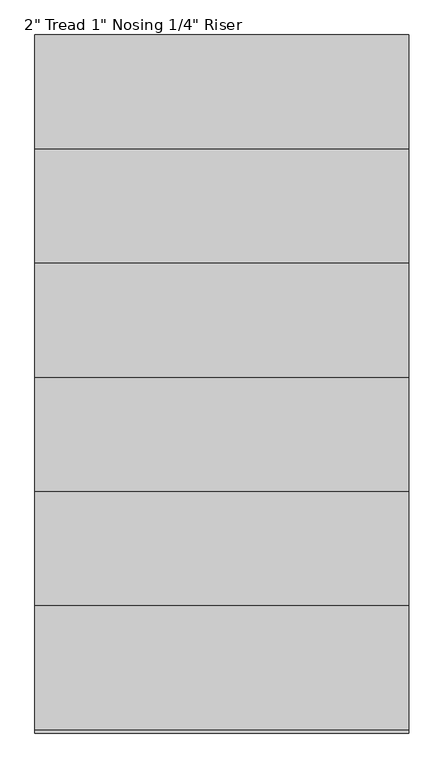
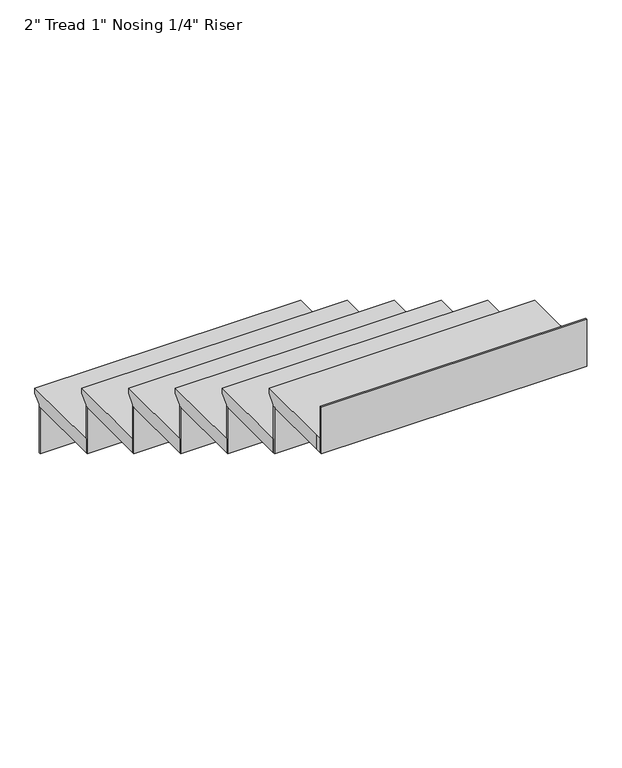
"""IFC4 building model written with IfcOpenShell, lengths in millimetres: stair flight geometry."""

from ifc_helpers import new_model, si_unit, origin, place, context, project, spatial, faceted_brep, source, transform, mapped, element, save


def stair_flight_23f0772b(model_context):
    return source(origin(), model_context, "Body", "Brep", [
        faceted_brep([(-11268.1522729, -356.3993654, 1301.75), (-11268.1522729, -356.3993654, 1320.8), (-10353.7522729, -356.3993654, 1320.8), (-10353.7522729, -356.3993654, 1301.75), (-11268.1522729, -381.7993654, 1276.35), (-10353.7522729, -381.7993654, 1276.35), (-11268.1522729, -661.1993654, 1320.8), (-10353.7522729, -661.1993654, 1320.8), (-10353.7522729, -381.7993654, 1270.0), (-10353.7522729, -661.1993654, 1270.0), (-11268.1522729, -661.1993654, 1270.0), (-11268.1522729, -381.7993654, 1270.0)], [[[0, 1, 2, 3]], [[4, 0, 3, 5]], [[2, 1, 6, 7]], [[8, 9, 10, 11]], [[2, 7, 9, 8, 5, 3]], [[8, 11, 4, 5]], [[6, 1, 0, 4, 11, 10]], [[7, 6, 10, 9]]]),
        faceted_brep([(-11268.1522729, -381.7993654, 1270.0), (-11268.1522729, -381.7993654, 1100.6666667), (-11268.1522729, -388.1493654, 1100.6666667), (-11268.1522729, -388.1493654, 1270.0), (-10353.7522729, -381.7993654, 1270.0), (-10353.7522729, -388.1493654, 1270.0), (-10353.7522729, -388.1493654, 1100.6666667), (-10353.7522729, -381.7993654, 1100.6666667)], [[[0, 1, 2, 3]], [[4, 5, 6, 7]], [[1, 0, 4, 7]], [[2, 1, 7, 6]], [[3, 2, 6, 5]], [[0, 3, 5, 4]]]),
        faceted_brep([(-11268.1522729, -661.1993654, 1439.3333333), (-11268.1522729, -661.1993654, 1270.0), (-11268.1522729, -667.5493654, 1270.0), (-11268.1522729, -667.5493654, 1439.3333333), (-10353.7522729, -661.1993654, 1439.3333333), (-10353.7522729, -667.5493654, 1439.3333333), (-10353.7522729, -667.5493654, 1270.0), (-10353.7522729, -661.1993654, 1270.0)], [[[0, 1, 2, 3]], [[4, 5, 6, 7]], [[1, 0, 4, 7]], [[2, 1, 7, 6]], [[3, 2, 6, 5]], [[0, 3, 5, 4]]]),
        faceted_brep([(-10353.7522729, -635.7993654, 1490.1333333), (-11268.1522729, -635.7993654, 1490.1333333), (-11268.1522729, -940.5993654, 1490.1333333), (-10353.7522729, -940.5993654, 1490.1333333), (-10353.7522729, -661.1993654, 1439.3333333), (-10353.7522729, -940.5993654, 1439.3333333), (-11268.1522729, -940.5993654, 1439.3333333), (-11268.1522729, -661.1993654, 1439.3333333), (-10353.7522729, -661.1993654, 1445.6833333), (-10353.7522729, -635.7993654, 1471.0833333), (-11268.1522729, -661.1993654, 1445.6833333), (-11268.1522729, -635.7993654, 1471.0833333)], [[[0, 1, 2, 3]], [[4, 5, 6, 7]], [[0, 3, 5, 4, 8, 9]], [[4, 7, 10, 8]], [[2, 1, 11, 10, 7, 6]], [[3, 2, 6, 5]], [[11, 1, 0, 9]], [[10, 11, 9, 8]]]),
        faceted_brep([(-11268.1522729, -940.5993654, 1608.6666667), (-11268.1522729, -940.5993654, 1439.3333333), (-11268.1522729, -946.9493654, 1439.3333333), (-11268.1522729, -946.9493654, 1608.6666667), (-10353.7522729, -940.5993654, 1608.6666667), (-10353.7522729, -946.9493654, 1608.6666667), (-10353.7522729, -946.9493654, 1439.3333333), (-10353.7522729, -940.5993654, 1439.3333333)], [[[0, 1, 2, 3]], [[4, 5, 6, 7]], [[1, 0, 4, 7]], [[2, 1, 7, 6]], [[3, 2, 6, 5]], [[0, 3, 5, 4]]]),
        faceted_brep([(-10353.7522729, -915.1993654, 1659.4666667), (-11268.1522729, -915.1993654, 1659.4666667), (-11268.1522729, -1219.9993654, 1659.4666667), (-10353.7522729, -1219.9993654, 1659.4666667), (-10353.7522729, -940.5993654, 1608.6666667), (-10353.7522729, -1219.9993654, 1608.6666667), (-11268.1522729, -1219.9993654, 1608.6666667), (-11268.1522729, -940.5993654, 1608.6666667), (-10353.7522729, -940.5993654, 1615.0166667), (-10353.7522729, -915.1993654, 1640.4166667), (-11268.1522729, -940.5993654, 1615.0166667), (-11268.1522729, -915.1993654, 1640.4166667)], [[[0, 1, 2, 3]], [[4, 5, 6, 7]], [[0, 3, 5, 4, 8, 9]], [[4, 7, 10, 8]], [[2, 1, 11, 10, 7, 6]], [[3, 2, 6, 5]], [[11, 1, 0, 9]], [[10, 11, 9, 8]]]),
        faceted_brep([(-11268.1522729, -1219.9993654, 1778.0), (-11268.1522729, -1219.9993654, 1608.6666667), (-11268.1522729, -1226.3493654, 1608.6666667), (-11268.1522729, -1226.3493654, 1778.0), (-10353.7522729, -1219.9993654, 1778.0), (-10353.7522729, -1226.3493654, 1778.0), (-10353.7522729, -1226.3493654, 1608.6666667), (-10353.7522729, -1219.9993654, 1608.6666667)], [[[0, 1, 2, 3]], [[4, 5, 6, 7]], [[1, 0, 4, 7]], [[2, 1, 7, 6]], [[3, 2, 6, 5]], [[0, 3, 5, 4]]]),
        faceted_brep([(-10353.7522729, -1194.5993654, 1828.8), (-11268.1522729, -1194.5993654, 1828.8), (-11268.1522729, -1499.3993654, 1828.8), (-10353.7522729, -1499.3993654, 1828.8), (-10353.7522729, -1219.9993654, 1778.0), (-10353.7522729, -1499.3993654, 1778.0), (-11268.1522729, -1499.3993654, 1778.0), (-11268.1522729, -1219.9993654, 1778.0), (-10353.7522729, -1219.9993654, 1784.35), (-10353.7522729, -1194.5993654, 1809.75), (-11268.1522729, -1219.9993654, 1784.35), (-11268.1522729, -1194.5993654, 1809.75)], [[[0, 1, 2, 3]], [[4, 5, 6, 7]], [[0, 3, 5, 4, 8, 9]], [[4, 7, 10, 8]], [[2, 1, 11, 10, 7, 6]], [[3, 2, 6, 5]], [[11, 1, 0, 9]], [[10, 11, 9, 8]]]),
        faceted_brep([(-11268.1522729, -1499.3993654, 1947.3333333), (-11268.1522729, -1499.3993654, 1778.0), (-11268.1522729, -1505.7493654, 1778.0), (-11268.1522729, -1505.7493654, 1947.3333333), (-10353.7522729, -1499.3993654, 1947.3333333), (-10353.7522729, -1505.7493654, 1947.3333333), (-10353.7522729, -1505.7493654, 1778.0), (-10353.7522729, -1499.3993654, 1778.0)], [[[0, 1, 2, 3]], [[4, 5, 6, 7]], [[1, 0, 4, 7]], [[2, 1, 7, 6]], [[3, 2, 6, 5]], [[0, 3, 5, 4]]]),
        faceted_brep([(-10353.7522729, -1473.9993654, 1998.1333333), (-11268.1522729, -1473.9993654, 1998.1333333), (-11268.1522729, -1778.7993654, 1998.1333333), (-10353.7522729, -1778.7993654, 1998.1333333), (-10353.7522729, -1499.3993654, 1947.3333333), (-10353.7522729, -1778.7993654, 1947.3333333), (-11268.1522729, -1778.7993654, 1947.3333333), (-11268.1522729, -1499.3993654, 1947.3333333), (-10353.7522729, -1499.3993654, 1953.6833333), (-10353.7522729, -1473.9993654, 1979.0833333), (-11268.1522729, -1499.3993654, 1953.6833333), (-11268.1522729, -1473.9993654, 1979.0833333)], [[[0, 1, 2, 3]], [[4, 5, 6, 7]], [[0, 3, 5, 4, 8, 9]], [[4, 7, 10, 8]], [[2, 1, 11, 10, 7, 6]], [[3, 2, 6, 5]], [[11, 1, 0, 9]], [[10, 11, 9, 8]]]),
        faceted_brep([(-11268.1522729, -2058.1993654, 2286.0), (-11268.1522729, -2058.1993654, 2116.6666667), (-11268.1522729, -2064.5493654, 2116.6666667), (-11268.1522729, -2064.5493654, 2286.0), (-10353.7522729, -2058.1993654, 2286.0), (-10353.7522729, -2064.5493654, 2286.0), (-10353.7522729, -2064.5493654, 2116.6666667), (-10353.7522729, -2058.1993654, 2116.6666667)], [[[0, 1, 2, 3]], [[4, 5, 6, 7]], [[1, 0, 4, 7]], [[2, 1, 7, 6]], [[3, 2, 6, 5]], [[0, 3, 5, 4]]]),
        faceted_brep([(-11268.1522729, -1778.7993654, 2116.6666667), (-11268.1522729, -1778.7993654, 1947.3333333), (-11268.1522729, -1785.1493654, 1947.3333333), (-11268.1522729, -1785.1493654, 2116.6666667), (-10353.7522729, -1778.7993654, 2116.6666667), (-10353.7522729, -1785.1493654, 2116.6666667), (-10353.7522729, -1785.1493654, 1947.3333333), (-10353.7522729, -1778.7993654, 1947.3333333)], [[[0, 1, 2, 3]], [[4, 5, 6, 7]], [[1, 0, 4, 7]], [[2, 1, 7, 6]], [[3, 2, 6, 5]], [[0, 3, 5, 4]]]),
        faceted_brep([(-10353.7522729, -1753.3993654, 2167.4666667), (-11268.1522729, -1753.3993654, 2167.4666667), (-11268.1522729, -2032.7993654, 2167.4666667), (-11268.1522729, -2058.1993654, 2167.4666667), (-10353.7522729, -2058.1993654, 2167.4666667), (-10353.7522729, -1778.7993654, 2116.6666667), (-10353.7522729, -2058.1993654, 2116.6666667), (-11268.1522729, -2058.1993654, 2116.6666667), (-11268.1522729, -2032.7993654, 2116.6666667), (-11268.1522729, -1778.7993654, 2116.6666667), (-10353.7522729, -1778.7993654, 2123.0166667), (-10353.7522729, -1753.3993654, 2148.4166667), (-11268.1522729, -1778.7993654, 2123.0166667), (-11268.1522729, -1753.3993654, 2148.4166667)], [[[0, 1, 2, 3, 4]], [[5, 6, 7, 8, 9]], [[0, 4, 6, 5, 10, 11]], [[5, 9, 12, 10]], [[2, 1, 13, 12, 9, 8]], [[3, 2, 8, 7]], [[4, 3, 7, 6]], [[13, 1, 0, 11]], [[12, 13, 11, 10]]]),
    ])


if __name__ == "__main__":
    model = new_model("IFC4")
    model_context = context("Model", 3, world=origin())
    ifc_project = project(units=[si_unit("LENGTHUNIT", "METRE", prefix="MILLI")], contexts=[model_context])
    site = spatial("IfcSite", under=ifc_project)
    building = spatial("IfcBuilding", under=site)
    placement = place(None, origin())
    stair_flight_shape = stair_flight_23f0772b(model_context)
    element("IfcStairFlight", 1, ObjectType="2\" Tread 1\" Nosing 1/4\" Riser", at=placement, inside=building, context=model_context, shape_type="MappedRepresentation", body=[
        mapped(stair_flight_shape, transform((0.0, 0.0, 0.0), x_axis=(1.0, 0.0, 0.0), y_axis=(0.0, 1.0, 0.0), z_axis=(0.0, 0.0, 1.0))),
    ])
    save(model, "model.ifc")
